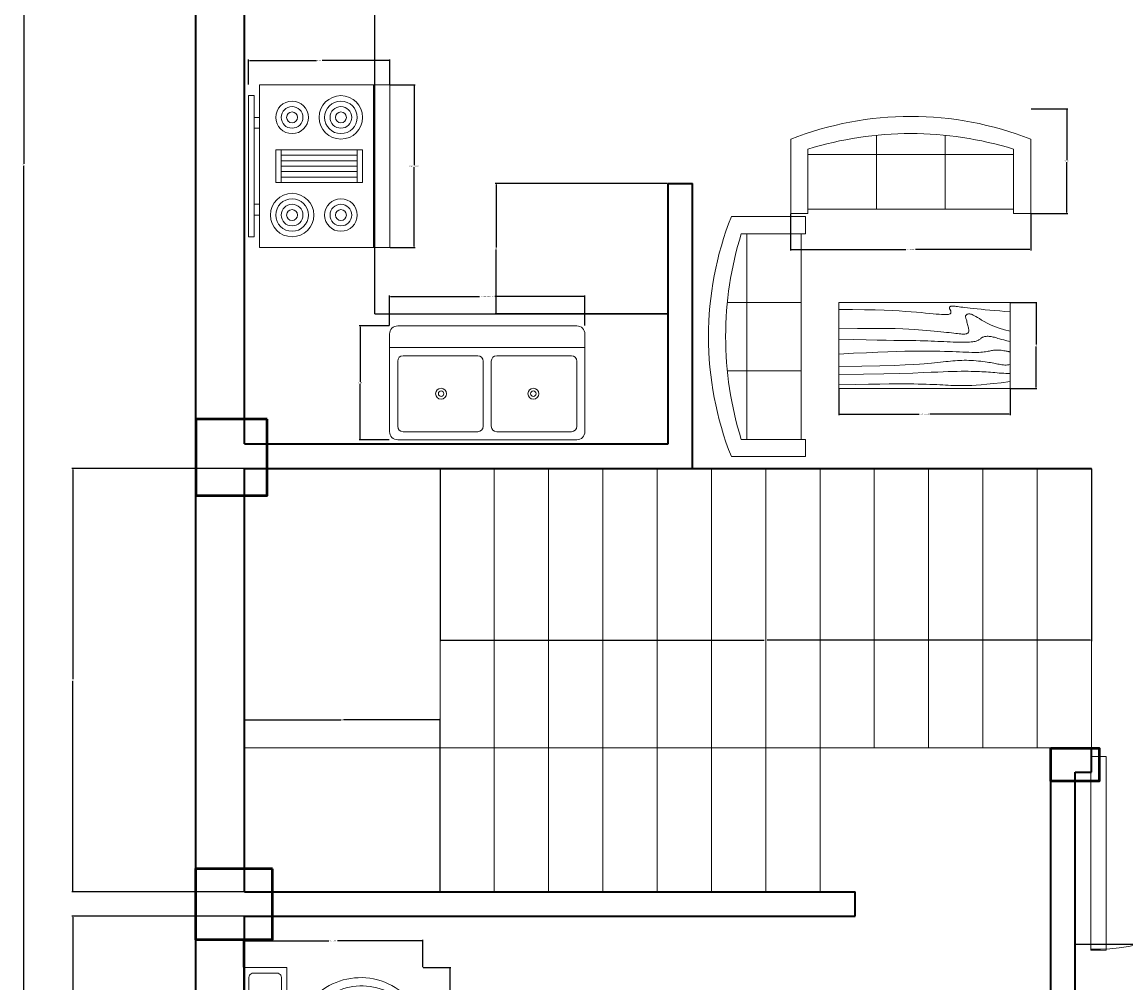
# Model space of a CAD drawing. Units: inches. Extents: x 50 to 2003, y -28 to 675.
# Tile 6 of 10: x 592 to 795, y 160 to 337. Entities that reach past the tile are written whole.
import ezdxf

# ---------------------------------------------------------------- set-up
doc = ezdxf.new("R2010")
doc.units = ezdxf.units.IN
for name, color, linetype, lineweight in [('A-ANNO-DIMS', 2, 'Continuous', 18), ('A-COLS', 1, 'Continuous', 50), ('A-DOOR', 4, 'Continuous', 18), ('A-EQPM', 8, 'Continuous', 18), ('A-FLOR-CASE', 32, 'Continuous', 25), ('A-FLOR-FIXT', 9, 'Continuous', 18), ('A-FLOR-STRS', 4, 'Continuous', 18), ('A-FURN', 8, 'Continuous', 18), ('A-WALL', 7, 'Continuous', 35)]:
    doc.layers.add(name, color=color, linetype=linetype, lineweight=lineweight)
doc.styles.get("Standard").update_dxf_attribs({"font": 'arial.ttf'})
doc.dimstyles.get("Standard").update_dxf_attribs({"dimtxt": 0.18, "dimasz": 0.18, "dimexe": 0.18, "dimexo": 0.0625, "dimgap": 0.09, "dimtad": 0, "dimtih": 1, "dimtoh": 1, "dimdec": 4, "dimzin": 0, "dimdsep": 46, "dimtxsty": 'Standard', "dimcen": 0.09, "dimadec": 0, "dimazin": 0, "dimtfac": 1, "dimtdec": 4, "dimtofl": 0, "dimtmove": 0, "dimatfit": 3, "dimfxl": 1, "dimtolj": 1, "dimtzin": 0, "dimarcsym": 0})

# ---------------------------------------------------------------- blocks, each defined once
blk = doc.blocks.new('Table - Rectangular Woodgrain 60 x 30 in.')
for p, q in [((0, 0), (0, -30)), ((60, 0), (0, 0)), ((60, -30), (60, 0)), ((0, -30), (60, -30))]:
    blk.add_line(p, q)
for points in [[(0, -2.4), (4.8155, -2.418), (9.0302, -2.4688), (12.709, -2.5477), (15.9167, -2.65), (18.7181, -2.7711), (21.1781, -2.9063), (23.3616, -3.0508), (25.3333, -3.2), (27.1477, -3.3495), (28.8172, -3.4958), (30.3437, -3.636), (31.7291, -3.7667), (32.9756, -3.8849), (34.0849, -3.9875), (35.059, -4.0714), (35.9, -4.1334), (36.6114, -4.1711), (37.2041, -4.1854), (37.6906, -4.1779), (38.0833, -4.15), (38.3948, -4.1034), (38.6375, -4.0396), (38.8239, -3.9602), (38.9666, -3.8667), (39.0764, -3.7608), (39.1573, -3.6448), (39.2116, -3.521), (39.2416, -3.3917), (39.2498, -3.2593), (39.2385, -3.1261), (39.21, -2.9944), (39.1666, -2.8667), (39.111, -2.7447), (39.0468, -2.6281), (38.978, -2.5163), (38.9083, -2.4083), (38.8418, -2.3035), (38.7823, -2.201), (38.7337, -2.1001), (38.7, -2), (38.6844, -1.9003), (38.6875, -1.8021), (38.7094, -1.707), (38.75, -1.6167), (38.8094, -1.5326), (38.8875, -1.4563), (38.9844, -1.3893), (39.1, -1.3333), (39.2351, -1.2896), (39.3937, -1.2583), (39.5804, -1.2396), (39.8, -1.2333), (40.057, -1.2396), (40.3562, -1.2583), (40.7023, -1.2896), (41.1, -1.3333), (41.5547, -1.3895), (42.0755, -1.4573), (42.6721, -1.5361), (43.3542, -1.625), (44.1316, -1.7233), (45.014, -1.8302), (46.0114, -1.9449), (47.1333, -2.0667), (48.3862, -2.1947), (49.7625, -2.3281), (51.2513, -2.4663), (52.8416, -2.6083), (54.5226, -2.7535), (56.2833, -2.9011), (58.1127, -3.0501), (60, -3.2)], [(0, -9.2), (6.5759, -9.0858), (11.9385, -9.0365), (16.2527, -9.0418), (19.6833, -9.0917), (22.3952, -9.1759), (24.5531, -9.2844), (26.322, -9.4069), (27.8666, -9.5333), (29.3241, -9.6553), (30.7203, -9.7719), (32.0532, -9.8837), (33.3208, -9.9917), (34.5213, -10.0965), (35.6526, -10.199), (36.7128, -10.2999), (37.7, -10.4), (38.6129, -10.4996), (39.4531, -10.5969), (40.223, -10.6895), (40.925, -10.775), (41.5613, -10.8512), (42.1344, -10.9156), (42.6465, -10.966), (43.1, -11), (43.4976, -11.0158), (43.8437, -11.0136), (44.143, -10.9942), (44.4, -10.9583), (44.6195, -10.9069), (44.8062, -10.8406), (44.9648, -10.7603), (45.1, -10.6667), (45.2155, -10.5598), (45.3114, -10.4365), (45.3871, -10.2929), (45.4416, -10.125), (45.4743, -9.929), (45.4844, -9.7011), (45.4709, -9.4371), (45.4333, -9.1333), (45.3716, -8.7883), (45.2896, -8.4104), (45.1919, -8.0107), (45.0833, -7.6), (44.9685, -7.1893), (44.8521, -6.7896), (44.7388, -6.4117), (44.6333, -6.0667), (44.54, -5.7628), (44.4614, -5.4979), (44.4001, -5.2675), (44.3583, -5.0667), (44.3384, -4.8909), (44.3427, -4.7354), (44.3736, -4.5956), (44.4333, -4.4667), (44.5236, -4.3453), (44.6427, -4.2333), (44.7884, -4.1339), (44.9583, -4.05), (45.1501, -3.9849), (45.3614, -3.9417), (45.59, -3.9234), (45.8333, -3.9333), (46.0915, -3.9749), (46.3734, -4.0531), (46.6906, -4.1736), (47.0542, -4.3417), (47.4756, -4.5629), (47.9661, -4.8427), (48.5372, -5.1866), (49.2, -5.6), (49.9676, -6.0844), (50.8594, -6.625), (51.8965, -7.2031), (53.1, -7.8), (54.491, -8.3969), (56.0906, -8.975), (57.9199, -9.5156), (60, -10)], [(0, -12.8), (5.1847, -12.9322), (9.6213, -13.0323), (13.3963, -13.1059), (16.5958, -13.1583), (19.3063, -13.1952), (21.614, -13.2219), (23.6054, -13.2439), (25.3666, -13.2667), (26.9728, -13.2947), (28.4531, -13.3281), (29.8256, -13.3663), (31.1083, -13.4083), (32.3191, -13.4535), (33.476, -13.501), (34.597, -13.5501), (35.7, -13.6), (36.7984, -13.6497), (37.8875, -13.6979), (38.9578, -13.743), (40, -13.7833), (41.0047, -13.8174), (41.9625, -13.8438), (42.864, -13.8607), (43.7, -13.8667), (44.4631, -13.8604), (45.1552, -13.8417), (45.7801, -13.8104), (46.3416, -13.7667), (46.8439, -13.7104), (47.2906, -13.6417), (47.6858, -13.5604), (48.0333, -13.4667), (48.3375, -13.3608), (48.6042, -13.2448), (48.8396, -13.121), (49.05, -12.9917), (49.2417, -12.8593), (49.4208, -12.7261), (49.5937, -12.5944), (49.7667, -12.4667), (49.9452, -12.3451), (50.1323, -12.2313), (50.3303, -12.1268), (50.5416, -12.0333), (50.7686, -11.9524), (51.0135, -11.8854), (51.2788, -11.8341), (51.5666, -11.8), (51.8785, -11.7843), (52.2116, -11.7865), (52.562, -11.8059), (52.926, -11.8417), (53.2998, -11.8931), (53.6795, -11.9594), (54.0614, -12.0397), (54.4416, -12.1333), (54.8223, -12.2401), (55.2293, -12.3625), (55.6942, -12.5037), (56.2489, -12.6667), (56.9251, -12.8547), (57.7545, -13.0708), (58.7689, -13.3182), (60, -13.6)], [(0, -18), (5.124, -17.7273), (9.6609, -17.5057), (13.6705, -17.3303), (17.2125, -17.1958), (20.3467, -17.0973), (23.1328, -17.0297), (25.6307, -16.9878), (27.9, -16.9667), (29.9928, -16.9617), (31.9302, -16.9703), (33.7254, -16.9907), (35.3917, -17.0208), (36.9423, -17.0588), (38.3906, -17.1026), (39.7499, -17.1503), (41.0333, -17.2), (42.2519, -17.2496), (43.4073, -17.2969), (44.4986, -17.3395), (45.525, -17.375), (46.4858, -17.4012), (47.3802, -17.4156), (48.2074, -17.416), (48.9667, -17.4), (49.6583, -17.3662), (50.2872, -17.3167), (50.8595, -17.2547), (51.3812, -17.1833), (51.8584, -17.1057), (52.2971, -17.025), (52.7034, -16.9443), (53.0833, -16.8667), (53.443, -16.7951), (53.789, -16.7313), (54.128, -16.6768), (54.4666, -16.6334), (54.8115, -16.6024), (55.1693, -16.5854), (55.5465, -16.5841), (55.95, -16.6), (56.3828, -16.6337), (56.8346, -16.6823), (57.2915, -16.7418), (57.7396, -16.8084), (58.165, -16.878), (58.5539, -16.9469), (58.8924, -17.0111), (59.1666, -17.0667), (59.3679, -17.1107), (59.5078, -17.1438), (59.6032, -17.1675), (59.6708, -17.1833), (59.7275, -17.193), (59.7901, -17.1979), (59.8753, -17.1998), (60, -17.2)], [(0, -22.4), (8.0098, -22.2501), (14.4094, -22.1011), (19.4168, -21.9535), (23.25, -21.8083), (26.1269, -21.6663), (28.2656, -21.5281), (29.884, -21.3947), (31.2, -21.2667), (32.3967, -21.1448), (33.5172, -21.0292), (34.5697, -20.9198), (35.5625, -20.8167), (36.5037, -20.7198), (37.4015, -20.6292), (38.2642, -20.5448), (39.1, -20.4667), (39.9164, -20.3951), (40.7187, -20.3313), (41.5117, -20.2768), (42.3, -20.2333), (43.0883, -20.2024), (43.8812, -20.1854), (44.6836, -20.1841), (45.5, -20.2), (46.3328, -20.234), (47.1747, -20.2844), (48.0163, -20.3488), (48.8479, -20.425), (49.66, -20.5106), (50.4429, -20.6031), (51.1872, -20.7004), (51.8833, -20.8), (52.5246, -20.8999), (53.1166, -20.9995), (53.6681, -21.0983), (54.1875, -21.1958), (54.6834, -21.2919), (55.1646, -21.3859), (55.6394, -21.4777), (56.1167, -21.5667), (56.6028, -21.6515), (57.0961, -21.7266), (57.5929, -21.7852), (58.0896, -21.8208), (58.5823, -21.8268), (59.0674, -21.7964), (59.5412, -21.723), (60, -21.6)], [(0, -25.2), (8.6355, -25.0504), (15.7026, -24.9031), (21.4049, -24.7606), (25.9458, -24.625), (29.529, -24.4988), (32.3578, -24.3844), (34.6359, -24.284), (36.5667, -24.2), (38.3213, -24.1341), (39.9417, -24.0854), (41.437, -24.0523), (42.8167, -24.0333), (44.0901, -24.0268), (45.2667, -24.0313), (46.3557, -24.0451), (47.3667, -24.0667), (48.309, -24.0947), (49.1928, -24.1287), (50.0284, -24.168), (50.826, -24.2125), (51.5959, -24.2617), (52.3483, -24.3151), (53.0935, -24.3725), (53.8417, -24.4334), (54.6009, -24.497), (55.3699, -24.561), (56.1454, -24.6226), (56.9239, -24.6792), (57.7021, -24.7279), (58.4764, -24.7662), (59.2435, -24.7911), (60, -24.8)], [(0, -28.8), (5.6867, -28.6681), (10.45, -28.5698), (14.407, -28.5012), (17.675, -28.4584), (20.3711, -28.4374), (22.6125, -28.4344), (24.5164, -28.4455), (26.2, -28.4667), (27.762, -28.4947), (29.2276, -28.5281), (30.6033, -28.5663), (31.8958, -28.6084), (33.1118, -28.6535), (34.2578, -28.7011), (35.3405, -28.7501), (36.3666, -28.8), (37.3443, -28.8497), (38.288, -28.8974), (39.2137, -28.9412), (40.1375, -28.9792), (41.0753, -29.0093), (42.0432, -29.0297), (43.0572, -29.0384), (44.1333, -29.0333), (45.2936, -29.0114), (46.5843, -28.9641), (48.0579, -28.8816), (49.7666, -28.7542), (51.7629, -28.5721), (54.0989, -28.3255), (56.8272, -28.0048), (60, -27.6)]]:
    blk.add_lwpolyline(points)
blk = doc.blocks.new('Sink-double - 36 in top')
for p, q in [((-18, -4), (18, -4)), ((-0.75, -18.5), (-0.75, -6.5)), ((0.75, -6.5), (0.75, -18.5))]:
    blk.add_line(p, q)
for points in [[(-16.5, 0), (16.5, 0)], [(-18, -19.5), (-18, -1.5)], [(18, -1.5), (18, -19.5)], [(-15.5, -5.5), (-1.75, -5.5)], [(1.75, -5.5), (15.5, -5.5)], [(-16.5, -18.5), (-16.5, -6.5)], [(16.5, -6.5), (16.5, -18.5)], [(-1.75, -19.5), (-15.5, -19.5)], [(15.5, -19.5), (1.75, -19.5)], [(16.5, -21), (-16.5, -21)]]:
    blk.add_lwpolyline(points)
for centre, radius in [((-8.5, -12.5), 1), ((-8.5, -12.5), 0.5), ((8.5, -12.5), 1), ((8.5, -12.5), 0.5)]:
    blk.add_circle(centre, radius)
for centre, radius, start, end in [((-16.5, -1.5), 1.5, 90, 180), ((16.5, -1.5), 1.5, 0, 90), ((-15.5, -6.5), 1, 90, 180), ((-1.75, -6.5), 1, 0, 90), ((1.75, -6.5), 1, 90, 180), ((15.5, -6.5), 1, 0, 90), ((-16.5, -19.5), 1.5, 180, 270), ((-15.5, -18.5), 1, 180, 270), ((-1.75, -18.5), 1, 270, 0), ((1.75, -18.5), 1, 180, 270), ((15.5, -18.5), 1, 270, 0), ((16.5, -19.5), 1.5, 270, 0)]:
    blk.add_arc(centre, radius, start, end)
blk = doc.blocks.new('Sofa - Roundback 7 ft.')
for p, q in [((-12.00002, -32.4421), (-12.00003, -6.5971)), ((11.99997, -32.4421), (11.99998, -6.5971)), ((-36.000027, -34), (-36.000027, -11.4696)), ((35.99998, -34), (35.99998, -11.4696)), ((-35.999844, -13.3819), (35.9998, -13.3819)), ((-36.000027, -32.4421), (35.99998, -32.4421))]:
    blk.add_line(p, q)
for points in [[(-36.000027, -34), (-42.000027, -34), (-42.000027, -8)], [(41.99998, -8), (41.99998, -34), (35.99998, -34)]]:
    blk.add_lwpolyline(points)
for centre, radius, start, end in [((0, -114.25), 114.25, 68.43141, 111.5686), ((-0.00001, -127.1968), 121.1968, 72.72033, 107.2797)]:
    blk.add_arc(centre, radius, start, end)
blk = doc.blocks.new('Range-Oven - 30 in top')
for p, q in [((0, -3), (30, -3)), ((12, -6), (18, -6)), ((13, -20), (13, -6)), ((14, -6), (14, -20)), ((15, -20), (15, -6)), ((16, -6), (16, -20)), ((17, -20), (17, -6)), ((18, -20), (12, -20)), ((6, -24), (6, -25)), ((8, -25), (8, -24)), ((22, -25), (22, -24)), ((24, -24), (24, -25))]:
    blk.add_line(p, q)
for points in [[(0, -24), (0, 0), (30, 0), (30, -24)], [(12, -21), (12, -5), (18, -5), (18, -21)], [(2, -26), (2, -25), (28, -25), (28, -26)]]:
    blk.add_lwpolyline(points, close=True)
for centre, radius in [((6, -9), 4), ((6, -9), 3), ((24, -9), 3), ((6, -9), 2), ((6, -9), 1), ((24, -9), 2), ((24, -9), 1), ((24, -18), 4), ((6, -18), 3), ((6, -18), 2), ((24, -18), 3), ((24, -18), 2), ((6, -18), 1), ((24, -18), 1)]:
    blk.add_circle(centre, radius)
blk = doc.blocks.new('Toilet - top')
for p, q in [((9.5, -6), (9.5, -2)), ((-8, -8.5), (-8, -8)), ((-7, -8), (-7, -9.5)), ((-4, -8), (-6, -14)), ((4, -8), (6, -14)), ((-10, -8.5), (-8, -8.5)), ((-10, -9.5), (-10, -8.5)), ((-7, -9.5), (-10, -9.5)), ((4, -14), (-4, -14))]:
    blk.add_line(p, q)
blk.add_lwpolyline([(10.5, -8), (10.5, 0), (-10.5, 0), (-10.5, -8)], close=True)
for points in [[(-9.5, -2), (-9.5, -6)], [(8.5, -1), (-8.5, -1)], [(-8.5, -7), (8.5, -7)]]:
    blk.add_lwpolyline(points)
for centre, radius, start, end in [((-8.62, -1.88), 0.884, 81.8699, 188.1301), ((8.62, -1.88), 0.884, 351.8699, 98.1301), ((-8.62, -6.12), 0.884, 171.8699, 278.1301), ((8.62, -6.12), 0.884, 261.8699, 8.1301), ((3.52, -21.58), 12.17, 141.4691, 247.9714), ((4.2, -21.82), 11.33, 136.3677, 238.9468), ((-3.52, -21.58), 12.17, 292.0284, 38.5307), ((-4.2, -21.82), 11.33, 301.053, 43.6321), ((0, -27.88), 4, 245.7318, 294.2682), ((0, -29), 4, 254.8605, 285.1395)]:
    blk.add_arc(centre, radius, start, end)
blk = doc.blocks.new('KITCHEN-COUNTER-L')
for q in [(0, 84), (54, 0)]:
    blk.add_line((0, 0), q)
blk = doc.blocks.new('DOOR-LEAF-36')
blk.add_lwpolyline([(35.71, 2.81), (35.71, 0), (0, 0), (0, 2.81)], close=True)
blk = doc.blocks.new('*D29')
at = {"layer": 'A-ANNO-DIMS', "color": 0, "lineweight": -2, "transparency": 16777216}
for p, q in [((632.4, 163.19), (632.4, 168.27)), ((632.58, 168.09), (648.14, 168.09)), ((665.26, 168.09), (649.7, 168.09)), ((665.44, 163.19), (665.44, 168.27))]:
    blk.add_line(p, q, dxfattribs=at)
at = {"layer": 'A-ANNO-DIMS', "color": 0, "transparency": 16777216}
for points in [[(632.58, 168.12), (632.58, 168.06), (632.4, 168.09)], [(665.26, 168.12), (665.26, 168.06), (665.44, 168.09)]]:
    blk.add_solid(points, dxfattribs=at)
at = {"layer": 'Defpoints', "color": 0, "transparency": 16777216}
for p in [(632.4, 168.09), (632.4, 163.13), (665.44, 163.13)]:
    blk.add_point(p, dxfattribs=at)
at = {"layer": 'A-ANNO-DIMS', "color": 0, "transparency": 16777216, "insert": (648.92, 168.09), "char_height": 0.18, "attachment_point": 5}
blk.add_mtext('\\A1;WC 33 TYP.', dxfattribs=at)
blk = doc.blocks.new('*D30')
at = {"layer": 'A-ANNO-DIMS', "color": 0, "lineweight": -2, "transparency": 16777216}
for p, q in [((665.51, 163.13), (670.58, 163.13)), ((670.4, 162.95), (670.4, 152.81)), ((670.4, 142.31), (670.4, 152.45)), ((665.51, 142.13), (670.58, 142.13))]:
    blk.add_line(p, q, dxfattribs=at)
at = {"layer": 'A-ANNO-DIMS', "color": 0, "transparency": 16777216}
for points in [[(670.37, 162.95), (670.43, 162.95), (670.4, 163.13)], [(670.37, 142.31), (670.43, 142.31), (670.4, 142.13)]]:
    blk.add_solid(points, dxfattribs=at)
at = {"layer": 'Defpoints', "color": 0, "transparency": 16777216}
for p in [(665.44, 163.13), (670.4, 163.13), (665.44, 142.13)]:
    blk.add_point(p, dxfattribs=at)
at = {"layer": 'A-ANNO-DIMS', "color": 0, "transparency": 16777216, "insert": (670.4, 152.63), "char_height": 0.18, "attachment_point": 5}
blk.add_mtext('\\A1;21 TYP.', dxfattribs=at)
blk = doc.blocks.new('*D37')
at = {"layer": 'A-ANNO-DIMS', "color": 0, "lineweight": -2, "transparency": 16777216}
for p, q in [((733.21, 302.02), (733.21, 295.26)), ((777.45, 302.02), (777.45, 295.26)), ((733.39, 295.44), (754.43, 295.44)), ((777.27, 295.44), (756.24, 295.44))]:
    blk.add_line(p, q, dxfattribs=at)
at = {"layer": 'A-ANNO-DIMS', "color": 0, "transparency": 16777216}
for points in [[(733.39, 295.47), (733.39, 295.41), (733.21, 295.44)], [(777.27, 295.47), (777.27, 295.41), (777.45, 295.44)]]:
    blk.add_solid(points, dxfattribs=at)
at = {"layer": 'Defpoints', "color": 0, "transparency": 16777216}
for p in [(733.21, 302.08), (777.45, 302.08), (777.45, 295.44)]:
    blk.add_point(p, dxfattribs=at)
at = {"layer": 'A-ANNO-DIMS', "color": 0, "transparency": 16777216, "insert": (755.33, 295.44), "char_height": 0.18, "attachment_point": 5}
blk.add_mtext('\\A1;SOFA 44 TYP.', dxfattribs=at)
blk = doc.blocks.new('*D38')
at = {"layer": 'A-ANNO-DIMS', "color": 0, "lineweight": -2, "transparency": 16777216}
for p, q in [((777.51, 321.39), (784.26, 321.39)), ((784.08, 321.21), (784.08, 311.92)), ((784.08, 302.26), (784.08, 311.55)), ((777.51, 302.08), (784.26, 302.08))]:
    blk.add_line(p, q, dxfattribs=at)
at = {"layer": 'A-ANNO-DIMS', "color": 0, "transparency": 16777216}
for points in [[(784.05, 321.21), (784.11, 321.21), (784.08, 321.39)], [(784.05, 302.26), (784.11, 302.26), (784.08, 302.08)]]:
    blk.add_solid(points, dxfattribs=at)
at = {"layer": 'Defpoints', "color": 0, "transparency": 16777216}
for p in [(777.45, 321.39), (784.08, 321.39), (777.45, 302.08)]:
    blk.add_point(p, dxfattribs=at)
at = {"layer": 'A-ANNO-DIMS', "color": 0, "transparency": 16777216, "insert": (784.08, 311.73), "char_height": 0.18, "attachment_point": 5}
blk.add_mtext('\\A1;19 TYP.', dxfattribs=at)
blk = doc.blocks.new('*D39')
at = {"layer": 'A-ANNO-DIMS', "color": 0, "lineweight": -2, "transparency": 16777216}
for p, q in [((659.42, 325.81), (664.04, 325.81)), ((663.86, 325.63), (663.86, 311)), ((663.86, 295.99), (663.86, 310.63)), ((659.42, 295.81), (664.04, 295.81))]:
    blk.add_line(p, q, dxfattribs=at)
at = {"layer": 'A-ANNO-DIMS', "color": 0, "transparency": 16777216}
for points in [[(663.83, 325.63), (663.89, 325.63), (663.86, 325.81)], [(663.83, 295.99), (663.89, 295.99), (663.86, 295.81)]]:
    blk.add_solid(points, dxfattribs=at)
at = {"layer": 'Defpoints', "color": 0, "transparency": 16777216}
for p in [(659.36, 325.81), (659.36, 295.81), (663.86, 295.81)]:
    blk.add_point(p, dxfattribs=at)
at = {"layer": 'A-ANNO-DIMS', "color": 0, "transparency": 16777216, "insert": (663.86, 310.81), "char_height": 0.18, "attachment_point": 5}
blk.add_mtext('\\A1;RANGE 30 TYP.', dxfattribs=at)
blk = doc.blocks.new('*D40')
at = {"layer": 'A-ANNO-DIMS', "color": 0, "lineweight": -2, "transparency": 16777216}
for p, q in [((633.36, 325.88), (633.36, 330.49)), ((633.54, 330.31), (645.83, 330.31)), ((659.18, 330.31), (646.89, 330.31)), ((659.36, 325.88), (659.36, 330.49))]:
    blk.add_line(p, q, dxfattribs=at)
at = {"layer": 'A-ANNO-DIMS', "color": 0, "transparency": 16777216}
for points in [[(633.54, 330.34), (633.54, 330.28), (633.36, 330.31)], [(659.18, 330.34), (659.18, 330.28), (659.36, 330.31)]]:
    blk.add_solid(points, dxfattribs=at)
at = {"layer": 'Defpoints', "color": 0, "transparency": 16777216}
for p in [(659.36, 330.31), (633.36, 325.81), (659.36, 325.81)]:
    blk.add_point(p, dxfattribs=at)
at = {"layer": 'A-ANNO-DIMS', "color": 0, "transparency": 16777216, "insert": (646.36, 330.31), "char_height": 0.18, "attachment_point": 5}
blk.add_mtext('\\A1;26 TYP.', dxfattribs=at)
blk = doc.blocks.new('*D43')
at = {"layer": 'A-ANNO-DIMS', "color": 0, "lineweight": -2, "transparency": 16777216}
for p, q in [((742.08, 269.81), (742.08, 264.95)), ((773.67, 269.81), (773.67, 264.95)), ((742.26, 265.13), (756.91, 265.13)), ((773.49, 265.13), (758.84, 265.13))]:
    blk.add_line(p, q, dxfattribs=at)
at = {"layer": 'A-ANNO-DIMS', "color": 0, "transparency": 16777216}
for points in [[(742.26, 265.16), (742.26, 265.1), (742.08, 265.13)], [(773.49, 265.16), (773.49, 265.1), (773.67, 265.13)]]:
    blk.add_solid(points, dxfattribs=at)
at = {"layer": 'Defpoints', "color": 0, "transparency": 16777216}
for p in [(742.08, 269.87), (773.67, 269.87), (773.67, 265.13)]:
    blk.add_point(p, dxfattribs=at)
at = {"layer": 'A-ANNO-DIMS', "color": 0, "transparency": 16777216, "insert": (757.88, 265.13), "char_height": 0.18, "attachment_point": 5}
blk.add_mtext('\\A1;LOW TABLE 32', dxfattribs=at)
blk = doc.blocks.new('*D44')
at = {"layer": 'A-ANNO-DIMS', "color": 0, "lineweight": -2, "transparency": 16777216}
for p, q in [((773.74, 285.67), (778.59, 285.67)), ((778.41, 285.49), (778.41, 277.95)), ((778.41, 270.05), (778.41, 277.59)), ((773.74, 269.87), (778.59, 269.87))]:
    blk.add_line(p, q, dxfattribs=at)
at = {"layer": 'A-ANNO-DIMS', "color": 0, "transparency": 16777216}
for points in [[(778.38, 285.49), (778.44, 285.49), (778.41, 285.67)], [(778.38, 270.05), (778.44, 270.05), (778.41, 269.87)]]:
    blk.add_solid(points, dxfattribs=at)
at = {"layer": 'Defpoints', "color": 0, "transparency": 16777216}
for p in [(773.67, 285.67), (778.41, 285.67), (773.67, 269.87)]:
    blk.add_point(p, dxfattribs=at)
at = {"layer": 'A-ANNO-DIMS', "color": 0, "transparency": 16777216, "insert": (778.41, 277.77), "char_height": 0.18, "attachment_point": 5}
blk.add_mtext('\\A1;16', dxfattribs=at)
blk = doc.blocks.new('*D47')
at = {"layer": 'A-ANNO-DIMS', "color": 0, "lineweight": -2, "transparency": 16777216}
for p, q in [((659.31, 281.45), (659.31, 286.97)), ((659.49, 286.79), (675.91, 286.79)), ((695.13, 286.79), (678.71, 286.79)), ((695.31, 281.45), (695.31, 286.97))]:
    blk.add_line(p, q, dxfattribs=at)
at = {"layer": 'A-ANNO-DIMS', "color": 0, "transparency": 16777216}
for points in [[(659.49, 286.82), (659.49, 286.76), (659.31, 286.79)], [(695.13, 286.82), (695.13, 286.76), (695.31, 286.79)]]:
    blk.add_solid(points, dxfattribs=at)
at = {"layer": 'Defpoints', "color": 0, "transparency": 16777216}
for p in [(695.31, 286.79), (659.31, 281.39), (695.31, 281.39)]:
    blk.add_point(p, dxfattribs=at)
at = {"layer": 'A-ANNO-DIMS', "color": 0, "transparency": 16777216, "insert": (677.31, 286.79), "char_height": 0.18, "attachment_point": 5}
blk.add_mtext('\\A1;DOUBLE SINK 36 TYP.', dxfattribs=at)
blk = doc.blocks.new('*D48')
at = {"layer": 'A-ANNO-DIMS', "color": 0, "lineweight": -2, "transparency": 16777216}
for p, q in [((659.25, 281.39), (653.73, 281.39)), ((653.91, 281.21), (653.91, 271.07)), ((653.91, 260.57), (653.91, 270.71)), ((659.25, 260.39), (653.73, 260.39))]:
    blk.add_line(p, q, dxfattribs=at)
at = {"layer": 'A-ANNO-DIMS', "color": 0, "transparency": 16777216}
for points in [[(653.88, 281.21), (653.94, 281.21), (653.91, 281.39)], [(653.88, 260.57), (653.94, 260.57), (653.91, 260.39)]]:
    blk.add_solid(points, dxfattribs=at)
at = {"layer": 'Defpoints', "color": 0, "transparency": 16777216}
for p in [(653.91, 281.39), (659.31, 281.39), (659.31, 260.39)]:
    blk.add_point(p, dxfattribs=at)
at = {"layer": 'A-ANNO-DIMS', "color": 0, "transparency": 16777216, "insert": (653.91, 270.89), "char_height": 0.18, "attachment_point": 5}
blk.add_mtext('\\A1;21 TYP.', dxfattribs=at)
blk = doc.blocks.new('*D75')
at = {"layer": 'A-ANNO-DIMS', "color": 0, "lineweight": -2, "transparency": 16777216}
for p, q in [((623.55, 618.62), (591.74, 618.62)), ((591.92, 618.44), (591.92, 311.25)), ((591.92, 3.7), (591.92, 310.89)), ((623.59, 3.52), (591.74, 3.52))]:
    blk.add_line(p, q, dxfattribs=at)
at = {"layer": 'A-ANNO-DIMS', "color": 0, "transparency": 16777216}
for points in [[(591.89, 618.44), (591.95, 618.44), (591.92, 618.62)], [(591.89, 3.7), (591.95, 3.7), (591.92, 3.52)]]:
    blk.add_solid(points, dxfattribs=at)
at = {"layer": 'Defpoints', "color": 0, "transparency": 16777216}
for p in [(591.92, 618.62), (623.62, 618.62), (623.65, 3.52)]:
    blk.add_point(p, dxfattribs=at)
at = {"layer": 'A-ANNO-DIMS', "color": 0, "transparency": 16777216, "insert": (591.92, 311.07), "char_height": 0.18, "attachment_point": 5}
blk.add_mtext('\\A1;615.1', dxfattribs=at)
blk = doc.blocks.new('*D86')
at = {"layer": 'A-ANNO-DIMS', "color": 0, "lineweight": -2, "transparency": 16777216}
for p, q in [((632.55, 172.62), (600.79, 172.62)), ((600.97, 172.44), (600.97, 139.8)), ((600.97, 106.8), (600.97, 139.44)), ((632.55, 106.62), (600.79, 106.62))]:
    blk.add_line(p, q, dxfattribs=at)
at = {"layer": 'A-ANNO-DIMS', "color": 0, "transparency": 16777216}
for points in [[(600.94, 172.44), (601, 172.44), (600.97, 172.62)], [(600.94, 106.8), (601, 106.8), (600.97, 106.62)]]:
    blk.add_solid(points, dxfattribs=at)
at = {"layer": 'Defpoints', "color": 0, "transparency": 16777216}
for p in [(600.97, 172.62), (632.62, 172.62), (632.62, 106.62)]:
    blk.add_point(p, dxfattribs=at)
at = {"layer": 'A-ANNO-DIMS', "color": 0, "transparency": 16777216, "insert": (600.97, 139.62), "char_height": 0.18, "attachment_point": 5}
blk.add_mtext('\\A1;66', dxfattribs=at)
blk = doc.blocks.new('*D87')
at = {"layer": 'A-ANNO-DIMS', "color": 0, "lineweight": -2, "transparency": 16777216}
for p, q in [((632.55, 255.12), (600.79, 255.12)), ((600.97, 254.94), (600.97, 216.3)), ((600.97, 177.3), (600.97, 215.94)), ((632.55, 177.12), (600.79, 177.12))]:
    blk.add_line(p, q, dxfattribs=at)
at = {"layer": 'A-ANNO-DIMS', "color": 0, "transparency": 16777216}
for points in [[(600.94, 254.94), (601, 254.94), (600.97, 255.12)], [(600.94, 177.3), (601, 177.3), (600.97, 177.12)]]:
    blk.add_solid(points, dxfattribs=at)
at = {"layer": 'Defpoints', "color": 0, "transparency": 16777216}
for p in [(600.97, 255.12), (632.62, 255.12), (632.62, 177.12)]:
    blk.add_point(p, dxfattribs=at)
at = {"layer": 'A-ANNO-DIMS', "color": 0, "transparency": 16777216, "insert": (600.97, 216.12), "char_height": 0.18, "attachment_point": 5}
blk.add_mtext('\\A1;78', dxfattribs=at)
blk = doc.blocks.new('*D90')
at = {"layer": 'A-ANNO-DIMS', "color": 0, "lineweight": -2, "transparency": 16777216}
for p, q in [((632.62, 177.18), (632.62, 208.95)), ((632.8, 208.77), (650.4, 208.77)), ((668.44, 208.77), (650.84, 208.77)), ((668.62, 177.18), (668.62, 208.95))]:
    blk.add_line(p, q, dxfattribs=at)
at = {"layer": 'A-ANNO-DIMS', "color": 0, "transparency": 16777216}
for points in [[(632.8, 208.8), (632.8, 208.74), (632.62, 208.77)], [(668.44, 208.8), (668.44, 208.74), (668.62, 208.77)]]:
    blk.add_solid(points, dxfattribs=at)
at = {"layer": 'Defpoints', "color": 0, "transparency": 16777216}
for p in [(668.62, 208.77), (632.62, 177.12), (668.62, 177.12)]:
    blk.add_point(p, dxfattribs=at)
at = {"layer": 'A-ANNO-DIMS', "color": 0, "transparency": 16777216, "insert": (650.62, 208.77), "char_height": 0.18, "attachment_point": 5}
blk.add_mtext('\\A1;36', dxfattribs=at)
blk = doc.blocks.new('*D91')
at = {"layer": 'A-ANNO-DIMS', "color": 0, "lineweight": -2, "transparency": 16777216}
for p, q in [((668.62, 255.06), (668.62, 223.29)), ((788.62, 255.06), (788.62, 223.29)), ((668.8, 223.47), (728.34, 223.47)), ((788.44, 223.47), (728.9, 223.47))]:
    blk.add_line(p, q, dxfattribs=at)
at = {"layer": 'A-ANNO-DIMS', "color": 0, "transparency": 16777216}
for points in [[(668.8, 223.5), (668.8, 223.44), (668.62, 223.47)], [(788.44, 223.5), (788.44, 223.44), (788.62, 223.47)]]:
    blk.add_solid(points, dxfattribs=at)
at = {"layer": 'Defpoints', "color": 0, "transparency": 16777216}
for p in [(668.62, 255.12), (788.62, 255.12), (668.62, 223.47)]:
    blk.add_point(p, dxfattribs=at)
at = {"layer": 'A-ANNO-DIMS', "color": 0, "transparency": 16777216, "insert": (728.62, 223.47), "char_height": 0.18, "attachment_point": 5}
blk.add_mtext('\\A1;120', dxfattribs=at)
blk = doc.blocks.new('*D94')
at = {"layer": 'A-ANNO-DIMS', "color": 0, "lineweight": -2, "transparency": 16777216}
for p, q in [((785.62, 199.06), (785.62, 167.29)), ((824.62, 199.06), (824.62, 167.29)), ((785.8, 167.47), (804.9, 167.47)), ((824.44, 167.47), (805.34, 167.47))]:
    blk.add_line(p, q, dxfattribs=at)
at = {"layer": 'A-ANNO-DIMS', "color": 0, "transparency": 16777216}
for points in [[(785.8, 167.5), (785.8, 167.44), (785.62, 167.47)], [(824.44, 167.5), (824.44, 167.44), (824.62, 167.47)]]:
    blk.add_solid(points, dxfattribs=at)
at = {"layer": 'Defpoints', "color": 0, "transparency": 16777216}
for p in [(785.62, 199.12), (824.62, 199.12), (785.62, 167.47)]:
    blk.add_point(p, dxfattribs=at)
at = {"layer": 'A-ANNO-DIMS', "color": 0, "transparency": 16777216, "insert": (805.12, 167.47), "char_height": 0.18, "attachment_point": 5}
blk.add_mtext('\\A1;39', dxfattribs=at)
blk = doc.blocks.new('*D95')
at = {"layer": 'A-ANNO-DIMS', "color": 0, "lineweight": -2, "transparency": 16777216}
for p, q in [((710.55, 307.62), (678.79, 307.62)), ((678.97, 307.44), (678.97, 295.8)), ((678.97, 283.8), (678.97, 295.44)), ((710.55, 283.62), (678.79, 283.62))]:
    blk.add_line(p, q, dxfattribs=at)
at = {"layer": 'A-ANNO-DIMS', "color": 0, "transparency": 16777216}
for points in [[(678.94, 307.44), (679, 307.44), (678.97, 307.62)], [(678.94, 283.8), (679, 283.8), (678.97, 283.62)]]:
    blk.add_solid(points, dxfattribs=at)
at = {"layer": 'Defpoints', "color": 0, "transparency": 16777216}
for p in [(678.97, 307.62), (710.62, 307.62), (710.62, 283.62)]:
    blk.add_point(p, dxfattribs=at)
at = {"layer": 'A-ANNO-DIMS', "color": 0, "transparency": 16777216, "insert": (678.97, 295.62), "char_height": 0.18, "attachment_point": 5}
blk.add_mtext('\\A1;24', dxfattribs=at)

msp = doc.modelspace()

# ---------------------------------------------------------------- linework, layer by layer
at = {"layer": 'A-COLS'}
for points in [[(636.7722, 264.2071), (623.6389, 264.2071), (623.6389, 250.1217), (636.7722, 250.1217)], [(781.1148, 203.5636), (790.0192, 203.5636), (790.0192, 197.4827), (781.1148, 197.4827)], [(637.7564, 181.343), (623.5919, 181.343), (623.5919, 168.3351), (637.7564, 168.3351)]]:
    msp.add_lwpolyline(points, close=True, dxfattribs=at)
at = {"layer": 'A-DOOR'}
msp.add_arc((789.3225, 201.8282), 35.3264, 268.663025, 356.673823, dxfattribs=at)
at = {"layer": 'A-FLOR-STRS'}
for p, q in [((668.6163, 177.1216), (668.6163, 255.1216)), ((678.6163, 177.1216), (678.6163, 255.1216)), ((688.6163, 177.1216), (688.6163, 255.1216)), ((698.6163, 177.1216), (698.6163, 255.1216)), ((708.6163, 177.1216), (708.6163, 255.1216)), ((718.6163, 177.1216), (718.6163, 255.1216)), ((728.6163, 177.1216), (728.6163, 255.1216)), ((738.6163, 177.1216), (738.6163, 255.1216)), ((748.6163, 203.6217), (748.6163, 255.1216)), ((758.6163, 203.6217), (758.6163, 255.1216)), ((768.6163, 203.6217), (768.6163, 255.1216)), ((778.6163, 203.6217), (778.6163, 255.1216)), ((788.6163, 203.6217), (788.6163, 255.1216)), ((632.6163, 203.6217), (788.6163, 203.6217))]:
    msp.add_line(p, q, dxfattribs=at)
at = {"layer": 'A-WALL'}
for p, q in [((623.6163, 3.6217), (623.6163, 618.6217)), ((632.6163, 259.6217), (632.6163, 367.6217)), ((710.6163, 259.6217), (710.6163, 307.6216)), ((710.6163, 307.6216), (715.1163, 307.6216)), ((715.1163, 255.1216), (715.1163, 307.6216)), ((632.6163, 259.6217), (710.6163, 259.6217)), ((632.6163, 255.1216), (788.6163, 255.1216)), ((632.6163, 177.1216), (632.6163, 255.1216)), ((781.1163, 3.6217), (781.1163, 203.6217)), ((788.6163, 199.1216), (788.6163, 203.6217)), ((785.6163, 55.1217), (785.6163, 199.1216)), ((785.6163, 199.1216), (788.6163, 199.1216)), ((632.6163, 177.1216), (745.1163, 177.1216)), ((745.1163, 172.6216), (745.1163, 177.1216)), ((632.6163, 172.6216), (745.1163, 172.6216)), ((632.6163, 106.6217), (632.6163, 172.6216))]:
    msp.add_line(p, q, dxfattribs=at)

# ---------------------------------------------------------------- block references
at = {"layer": 'A-DOOR', "rotation": 269.9999999999999}
msp.add_blockref('DOOR-LEAF-36', (788.5243, 202.0595), dxfattribs=at)
at = {"layer": 'A-EQPM', "rotation": 270}
msp.add_blockref('Range-Oven - 30 in top', (659.3563, 325.8131), dxfattribs=at)
at = {"layer": 'A-FLOR-CASE'}
msp.add_blockref('KITCHEN-COUNTER-L', (656.6163, 283.6216), dxfattribs=at)
at = {"layer": 'A-FLOR-FIXT'}
msp.add_blockref('Sink-double - 36 in top', (677.3109, 281.3899), dxfattribs=at)
at = {"layer": 'A-FLOR-FIXT', "rotation": 89.99999999999999}
msp.add_blockref('Toilet - top', (632.3978, 152.6305), dxfattribs=at)
at = {"layer": 'A-FURN', "xscale": 0.5266228823023269, "yscale": 0.5266228823023269, "zscale": 0.5266228823023269}
for name, p in [('Sofa - Roundback 7 ft.', (755.3307, 319.9839)), ('Table - Rectangular Woodgrain 60 x 30 in.', (742.077, 285.6669))]:
    msp.add_blockref(name, p, dxfattribs=at)
at = {"layer": 'A-FURN', "xscale": 0.5266228823023269, "yscale": 0.5266228823023269, "zscale": 0.5266228823023269, "rotation": 90}
msp.add_blockref('Sofa - Roundback 7 ft.', (718.0699, 279.404), dxfattribs=at)

# ---------------------------------------------------------------- dimensions: what is measured, and where the dimension line sits
at = {"layer": 'A-ANNO-DIMS'}
for base, p1, p2, angle, override, picture, middle in [((591.9232, 618.6217), (623.6536, 3.5196), (623.6163, 618.6217), 90, {"dimdec": 1, "dimlfac": 1, "dimrnd": 0, "dimzin": 0, "dimdsep": 46, "dimlunit": 2}, '*D75', (591.9232, 311.0706)), ((678.9663, 307.6216), (710.6163, 283.6216), (710.6163, 307.6216), 90, {"dimdec": 0, "dimlfac": 1, "dimrnd": 0, "dimzin": 0, "dimdsep": 46, "dimlunit": 2}, '*D95', (678.9663, 295.6216)), ((778.414, 285.6669), (773.6744, 269.8682), (773.6744, 285.6669), 90, {"dimdec": 0, "dimlfac": 1, "dimrnd": 0, "dimzin": 0, "dimdsep": 46, "dimlunit": 2}, '*D44', (778.414, 277.7676)), ((600.9663, 255.1216), (632.6163, 177.1216), (632.6163, 255.1216), 90, {"dimdec": 0, "dimlfac": 1, "dimrnd": 0, "dimzin": 0, "dimdsep": 46, "dimlunit": 2}, '*D87', (600.9663, 216.1216)), ((668.6163, 223.4717), (788.6163, 255.1216), (668.6163, 255.1216), 180, {"dimdec": 0, "dimlfac": 1, "dimrnd": 0, "dimzin": 0, "dimdsep": 46, "dimlunit": 2}, '*D91', (728.6163, 223.4717)), ((785.6163, 167.4717), (824.6163, 199.1216), (785.6163, 199.1216), 180, {"dimdec": 0, "dimlfac": 1, "dimrnd": 0, "dimzin": 0, "dimdsep": 46, "dimlunit": 2}, '*D94', (805.1163, 167.4717)), ((600.9663, 172.6216), (632.6163, 106.6217), (632.6163, 172.6216), 90, {"dimdec": 0, "dimlfac": 1, "dimrnd": 0, "dimzin": 0, "dimdsep": 46, "dimlunit": 2}, '*D86', (600.9663, 139.6216))]:
    dim = msp.add_linear_dim(base=base, p1=p1, p2=p2, angle=angle, dimstyle='Standard', override=override, dxfattribs=at)
    dim.commit()
    dim.dimension.update_dxf_attribs({"geometry": picture, "text_midpoint": middle})
for base, p1, p2, text, picture, middle in [((659.3563, 330.3131), (633.3563, 325.8131), (659.3563, 325.8131), '<> TYP.', '*D40', (646.3563, 330.3131)), ((777.4488, 295.4433), (733.2125, 302.0787), (777.4488, 302.0787), 'SOFA <> TYP.', '*D37', (755.3307, 295.4433)), ((695.3109, 286.7899), (659.3109, 281.3899), (695.3109, 281.3899), 'DOUBLE SINK <> TYP.', '*D47', (677.3109, 286.7899)), ((773.6744, 265.1286), (742.077, 269.8682), (773.6744, 269.8682), 'LOW TABLE <>', '*D43', (757.8757, 265.1286))]:
    dim = msp.add_linear_dim(base=base, p1=p1, p2=p2, text=text, dimstyle='Standard', override={"dimdec": 0, "dimlfac": 1, "dimrnd": 0, "dimzin": 0, "dimdsep": 46, "dimlunit": 2}, dxfattribs=at)
    dim.commit()
    dim.dimension.update_dxf_attribs({"geometry": picture, "text_midpoint": middle})
for base, p1, p2, angle, text, picture, middle in [((663.8563, 295.8131), (659.3563, 325.8131), (659.3563, 295.8131), 270, 'RANGE <> TYP.', '*D39', (663.8563, 310.8131)), ((784.0843, 321.3882), (777.4488, 302.0787), (777.4488, 321.3882), 90, '<> TYP.', '*D38', (784.0843, 311.7335)), ((653.9109, 281.3899), (659.3109, 260.3899), (659.3109, 281.3899), 90, '<> TYP.', '*D48', (653.9109, 270.8899)), ((632.3978, 168.0874), (665.4441, 163.1305), (632.3978, 163.1305), 180, 'WC <> TYP.', '*D29', (648.9209, 168.0874)), ((670.401, 163.1305), (665.4441, 142.1305), (665.4441, 163.1305), 90, '<> TYP.', '*D30', (670.401, 152.6305))]:
    dim = msp.add_linear_dim(base=base, p1=p1, p2=p2, angle=angle, text=text, dimstyle='Standard', override={"dimdec": 0, "dimlfac": 1, "dimrnd": 0, "dimzin": 0, "dimdsep": 46, "dimlunit": 2}, dxfattribs=at)
    dim.commit()
    dim.dimension.update_dxf_attribs({"geometry": picture, "text_midpoint": middle})
dim = msp.add_linear_dim(base=(668.6163, 208.7716), p1=(632.6163, 177.1216), p2=(668.6163, 177.1216), dimstyle='Standard', override={"dimdec": 0, "dimlfac": 1, "dimrnd": 0, "dimzin": 0, "dimdsep": 46, "dimlunit": 2}, dxfattribs=at)
dim.commit()
dim.dimension.update_dxf_attribs({"geometry": '*D90', "text_midpoint": (650.6163, 208.7716)})

doc.saveas('drawing.dxf')
